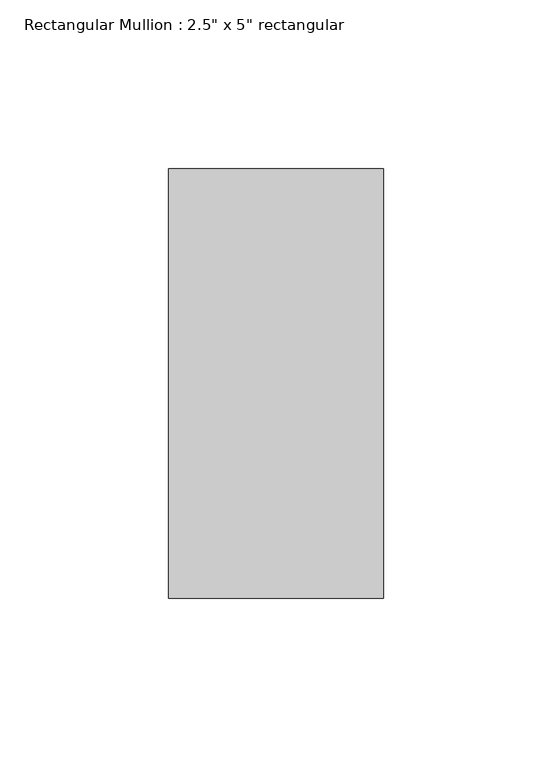
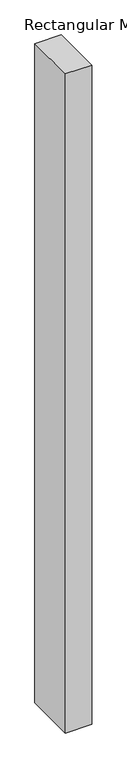
"""IFC4 building model written with IfcOpenShell, lengths in millimetres: member geometry."""

from ifc_helpers import new_model, si_unit, frame, origin, place, context, project, spatial, polyline, outline, extrude, source, transform, mapped, element, save


def member_bdb631d2(model_context):
    return source(origin(), model_context, "Body", "SweptSolid", [
        extrude(outline(polyline([(0.0, 63.5), (0.0, -63.5), (-63.5, -63.5), (-63.5, 63.5), (0.0, 63.5)])), frame((0.0, 0.0, -1676.3357893), z_axis=(0.0, 0.0, 1.0), x_axis=(1.0, 0.0, 0.0)), (0.0, 0.0, 1.0), 1676.3357893),
    ])


if __name__ == "__main__":
    model = new_model("IFC4")
    model_context = context("Model", 3, world=origin())
    ifc_project = project(units=[si_unit("LENGTHUNIT", "METRE", prefix="MILLI")], contexts=[model_context])
    site = spatial("IfcSite", under=ifc_project)
    building = spatial("IfcBuilding", under=site)
    placement = place(None, origin())
    member_shape = member_bdb631d2(model_context)
    element("IfcMember", 1, ObjectType="Rectangular Mullion : 2.5\" x 5\" rectangular", at=placement, inside=building, context=model_context, shape_type="MappedRepresentation", body=[
        mapped(member_shape, transform((0.0, 0.0, 0.0), x_axis=(1.0, 0.0, 0.0), y_axis=(0.0, 1.0, 0.0), z_axis=(0.0, 0.0, 1.0))),
    ])
    save(model, "model.ifc")

# Revit data of these elements
# Type "Rectangular Mullion : 2.5\" x 5\" rectangular"
#   built-in parameter 1007304 = 0.416667 (stored number, unit not read)
#   built-in parameter 1007301 = 0.104167 (stored number, unit not read)
#   built-in parameter 1007300 = 0.104167 (stored number, unit not read)
# Element 1 (IfcMember, "Rectangular Mullion : 2.5\" x 5\" rectangular")
#   Materials on its faces: "Aluminum"
# Materials
#   "Aluminum": class "Metal", colour RGB 247 247 247, transparency 0, Description = "Aluminum 6061", Cost = 0
